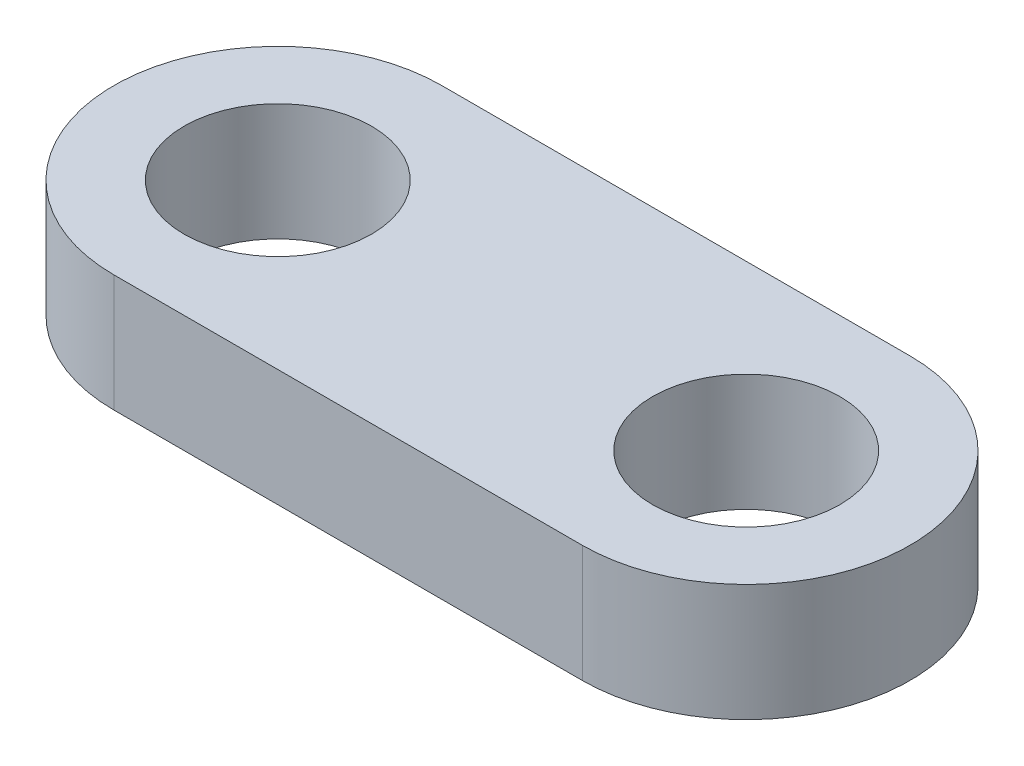
SolidWorks part; units mm, degrees
material "Plain Carbon Steel"
ref_plane "Front Plane" through (0, 0, 0) normal (0, 0, 1) x (1, 0, 0)
ref_plane "Top Plane" through (0, 0, 0) normal (0, 1, 0) x (1, 0, 0)
ref_plane "Right Plane" through (0, 0, 0) normal (1, 0, 0) x (0, 0, -1)
sketch "Link Profile Sketch" plane through (0, 0, 0) normal (0, 1, 0) x (1, 0, 0)
  line L0 (-431.1168, 0) -> (21124.725, 0) construction
  line L1 (0, -431.1168) -> (0, 21124.725) construction
  line L2 (-10, 0) -> (10, 0) construction
  line L3 (-10, 7) -> (10, 7)
  line L4 (-10, -7) -> (10, -7)
  arc A0 (-10, 7) -> (-10, -7) centre (-10, 0) ccw
  arc A1 (10, -7) -> (10, 7) centre (10, 0) ccw
  point P7 (0, 0)
  dimension "D1" = 7
  dimension "D2" = 20
  dimension "D3" = 10
extrude "Link Plate" add sketch "Link Profile Sketch" along normal mid plane 5
sketch "Hole Sketch" plane through (0, 0, 0) normal (0, 1, 0) x (1, 0, 0)
  circle A1 centre (10, 0) radius 4
  circle A2 centre (-10, 0) radius 4
  dimension "D1" = 8
  dimension "D2" = 8
extrude "Through Holes 2xØ8" cut sketch "Hole Sketch" against normal mid plane 5
